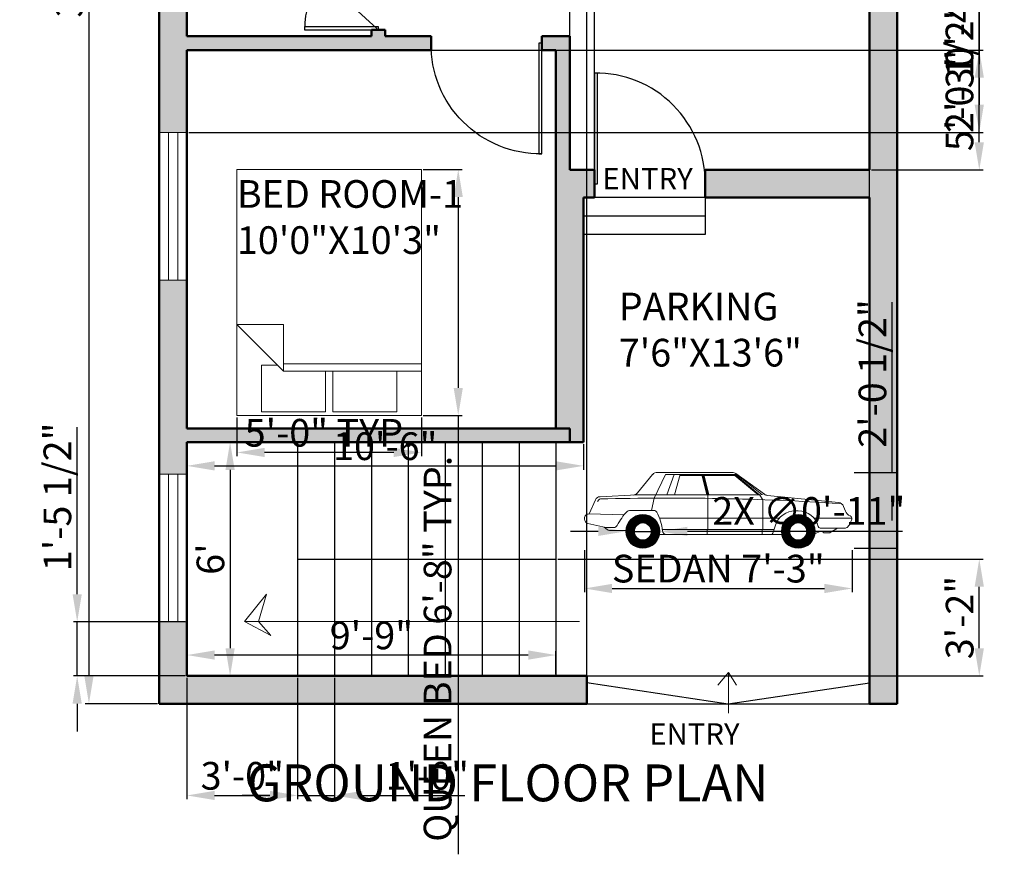
# Model space of a CAD drawing. Units: inches. Extents: x 66818 to 67138, y 29633 to 30215.
# Tile 1 of 2: x 66818 to 67138, y 29633 to 29904. Entities that reach past the tile are written whole.
import ezdxf

# ---------------------------------------------------------------- set-up
doc = ezdxf.new("R2010")
doc.units = ezdxf.units.IN
for name, color, linetype, lineweight in [('A-ANNO-DIMS', 2, 'Continuous', 18), ('A-ANNO-SYMB', 7, 'Continuous', 18), ('A-ANNO-TEXT', 7, 'Continuous', 25), ('A-AREA-IDEN', 7, 'Continuous', 25), ('A-DOOR', 3, 'Continuous', 25), ('A-FLOR-STRS', 7, 'Continuous', 25), ('A-FURN', 8, 'Continuous', 18), ('A-GLAZ', 4, 'Continuous', 18), ('A-SITE-PARK', 9, 'Continuous', 13), ('A-WALL', 7, 'Continuous', 50)]:
    doc.layers.add(name, color=color, linetype=linetype, lineweight=lineweight)
doc.layers.add('A-WALL-PATT', color=251, linetype='Continuous', lineweight=13, true_color=0x636466)
doc.styles.get("Standard").update_dxf_attribs({"font": 'arial.ttf'})
doc.dimstyles.new('ISO-25', dxfattribs={"dimtxt": 9, "dimasz": 9, "dimexe": 1.25, "dimexo": 0.625, "dimtad": 1, "dimdec": 1, "dimrnd": 9, "dimlunit": 3, "dimtxsty": 'Standard', "dimcen": 2.5, "dimadec": 0, "dimazin": 0, "dimtfac": 1, "dimtdec": 1, "dimtmove": 0, "dimatfit": 3, "dimfxl": 1, "dimarcsym": 0})

# ---------------------------------------------------------------- blocks, each defined once
blk = doc.blocks.new('*D1')
at = {"layer": 'A-ANNO-DIMS', "color": 0, "lineweight": -2, "transparency": 16777216}
for p, q in [((66872.23, 29766.29), (66872.23, 29757.97)), ((67001.23, 29766.29), (67001.23, 29757.97)), ((66881.23, 29759.22), (66992.23, 29759.22))]:
    blk.add_line(p, q, dxfattribs=at)
at = {"layer": 'A-ANNO-DIMS', "color": 0, "transparency": 16777216}
for points in [[(66881.23, 29760.72), (66881.23, 29757.72), (66872.23, 29759.22)], [(66992.23, 29760.72), (66992.23, 29757.72), (67001.23, 29759.22)]]:
    blk.add_solid(points, dxfattribs=at)
at = {"layer": 'Defpoints', "color": 0, "transparency": 16777216}
for p in [(66872.23, 29766.91), (67001.23, 29766.91), (67001.23, 29759.22)]:
    blk.add_point(p, dxfattribs=at)
at = {"layer": 'A-ANNO-DIMS', "color": 0, "transparency": 16777216, "insert": (66936.73, 29764.44), "char_height": 9, "attachment_point": 5}
blk.add_mtext('10\'-6"', dxfattribs=at)
blk = doc.blocks.new('*D2')
at = {"layer": 'A-ANNO-DIMS', "color": 0, "lineweight": -2, "transparency": 16777216}
for p, q in [((66872.85, 29766.91), (66887.51, 29766.91)), ((66886.26, 29757.91), (66886.26, 29699.91)), ((66872.85, 29690.91), (66887.51, 29690.91))]:
    blk.add_line(p, q, dxfattribs=at)
at = {"layer": 'A-ANNO-DIMS', "color": 0, "transparency": 16777216}
for points in [[(66884.76, 29757.91), (66887.76, 29757.91), (66886.26, 29766.91)], [(66884.76, 29699.91), (66887.76, 29699.91), (66886.26, 29690.91)]]:
    blk.add_solid(points, dxfattribs=at)
at = {"layer": 'Defpoints', "color": 0, "transparency": 16777216}
for p in [(66872.23, 29766.91), (66872.23, 29690.91), (66886.26, 29690.91)]:
    blk.add_point(p, dxfattribs=at)
at = {"layer": 'A-ANNO-DIMS', "color": 0, "transparency": 16777216, "insert": (66881.04, 29728.91), "char_height": 9, "attachment_point": 5, "rotation": 90}
blk.add_mtext("6'", dxfattribs=at)
blk = doc.blocks.new('*D3')
at = {"layer": 'A-ANNO-DIMS', "color": 0, "lineweight": -2, "transparency": 16777216}
for p, q in [((66872.23, 29691.54), (66872.23, 29698.96)), ((66983.23, 29697.71), (66881.23, 29697.71)), ((66992.23, 29691.54), (66992.23, 29698.96))]:
    blk.add_line(p, q, dxfattribs=at)
at = {"layer": 'A-ANNO-DIMS', "color": 0, "transparency": 16777216}
for points in [[(66881.23, 29699.21), (66881.23, 29696.21), (66872.23, 29697.71)], [(66983.23, 29699.21), (66983.23, 29696.21), (66992.23, 29697.71)]]:
    blk.add_solid(points, dxfattribs=at)
at = {"layer": 'Defpoints', "color": 0, "transparency": 16777216}
for p in [(66872.23, 29697.71), (66872.23, 29690.91), (66992.23, 29690.91)]:
    blk.add_point(p, dxfattribs=at)
at = {"layer": 'A-ANNO-DIMS', "color": 0, "transparency": 16777216, "insert": (66932.23, 29702.93), "char_height": 9, "attachment_point": 5}
blk.add_mtext('9\'-9"', dxfattribs=at)
blk = doc.blocks.new('Bed - Queen')
for p, q in [((0, -80.00003), (0, 0)), ((0, 0), (59.99999, 0)), ((59.99999, 0), (59.99999, -80.00003)), ((7.99999, -1.2), (28.79998, -1.2)), ((7.99999, -14.4), (7.99999, -1.2)), ((28.79998, -1.2), (28.79998, -14.4)), ((31.19999, -1.2), (51.99999, -1.2)), ((31.19999, -14.4), (31.19999, -1.2)), ((51.99999, -1.2), (51.99999, -16.4)), ((0, -14.4), (44.8, -14.4)), ((59.99999, -29.6), (44.8, -14.4)), ((44.8, -14.4), (44.8, -29.6)), ((44.8, -16.8), (0, -16.8)), ((51.99999, -16.4), (46.79936, -16.4)), ((44.8, -29.6), (59.99999, -29.6)), ((59.99999, -80.00003), (0, -80.00003))]:
    blk.add_line(p, q)
blk = doc.blocks.new('Car - sedan  side')
for p, q in [((-139.53, 35.99), (-129.64, 47.91)), ((-128.57, 32.64), (-121.22, 48.02)), ((-77.81, 49.34), (-126.58, 49.34)), ((-74.7, 48.02), (-121.22, 48.02)), ((-120.32, 34.67), (-115.67, 48.02)), ((-115.4, 34.67), (-111.74, 48.02)), ((-97.55, 47.3), (-111.94, 47.3)), ((-94.41, 34.67), (-97.73, 48.02)), ((-93.72, 34.67), (-97.04, 48.02)), ((-93.03, 34.67), (-96.34, 48.02)), ((-76.26, 47.3), (-96.16, 47.3)), ((-61.08, 34.66), (-76.26, 47.3)), ((-60.02, 34.65), (-76.07, 48.02)), ((-56.87, 35.13), (-75.48, 48.59)), ((-58.54, 34.93), (-74.99, 48.02)), ((-140.23, 34.67), (-163.88, 33.56)), ((-62.28, 34.67), (-140.23, 34.67)), ((-130.39, 24.63), (-128.57, 32.64)), ((-93.72, 19.62), (-93.72, 34.67)), ((-62.28, 34.67), (-60.02, 34.65)), ((-60.02, 34.65), (-58.54, 34.93)), ((-57.97, 31.61), (-60.02, 34.65)), ((-57.21, 35.38), (-58.54, 34.93)), ((-54.93, 34.4), (-8.75, 29.8)), ((-170.93, 22.32), (-166.81, 31.56)), ((-164.57, 31.6), (-165.48, 30.35)), ((-57.97, 19.62), (-57.97, 31.61)), ((-4.21, 24.18), (-5.42, 27.27)), ((-174, 19.51), (-174, 18.91)), ((-148.26, 21.7), (-171.11, 22.33)), ((-128.78, 24.63), (-144.79, 24.63)), ((-47.2, 19.62), (-125.23, 19.62)), ((-93.72, 12.14), (-93.72, 19.62)), ((-57.97, 12.14), (-57.97, 19.62)), ((-36.97, 24.38), (-34.94, 24.38)), ((0, 19.62), (-24.7, 19.62)), ((-160.12, 13.48), (-171.81, 16.16)), ((-159.22, 12.14), (-161.08, 13.7)), ((-155.01, 13.48), (-160.12, 13.48)), ((-51.4, 9.89), (-49.69, 15.14)), ((-4.23, 13.19), (-20.72, 13.19)), ((-9.5, 13.19), (-14.1, 10.2)), ((-3.22, 13.59), (-1.77, 14.97)), ((-147.03, 11.6), (-157.73, 11.6)), ((-120.62, 9.03), (-125.23, 9.03)), ((-50.67, 12.14), (-123.32, 12.14)), ((-45.76, 9.03), (-120.62, 9.03)), ((-94.21, 9.03), (-94.21, 12.14)), ((-58.39, 9.03), (-58.39, 12.14)), ((-20.36, 11.06), (-24.06, 9.44)), ((-18.83, 10.42), (-19.11, 10.76)), ((-14.68, 10.03), (-18.01, 10.03))]:
    blk.add_line(p, q)
at = {"const_width": 5.49}
for points in [[(-127.8, 11, -1), (-144.3, 11, -1)], [(-26.69, 11, -1), (-43.19, 11, -1)]]:
    blk.add_lwpolyline(points, format="xyb", close=True, dxfattribs=at)
for centre, radius in [((-136.05, 11), 11), ((-34.94, 11), 11), ((-136.05, 11), 5.51), ((-34.94, 11), 5.51)]:
    blk.add_circle(centre, radius)
for centre, radius, start, end in [((-126.58, 45.38), 3.97, 90, 140.30288), ((-77.81, 45.38), 3.97, 54.13504, 90), ((-163.72, 30.18), 3.38, 92.68266, 155.97362), ((-163.62, 30.91), 1.17, 91.49105, 143.95527), ((-118.51, -1702.12), 1734.79, 86.34698, 91.49105), ((-142.58, 38.53), 3.97, 272.68265, 320.30288), ((-54.54, 38.35), 3.97, 234.13503, 264.31231), ((-9.15, 25.82), 4, 21.31069, 84.3123), ((-171.18, 19.51), 2.82, 88.41927, 180), ((-118.09, -2.78), 38.85, 136.3964, 152.90974), ((-144.79, 22.64), 1.98, 90, 136.3964), ((-128.78, 22.64), 1.98, 28.1371, 90), ((-157.14, 7.48), 34.14, 6.51354, 28.1371), ((-36.97, 11), 13.38, 90, 161.97316), ((-34.94, 11), 13.38, 13.58642, 90), ((0.9, 26.18), 5.49, 201.3107, 247.70484), ((-1.92, 19.3), 1.94, 325.37436, 67.70485), ((-171.18, 18.91), 2.82, 180, 257.09053), ((-155.01, 16.1), 2.62, 270, 332.90974), ((-20.72, 14.43), 1.24, 193.58641, 270), ((-4.23, 14.65), 1.46, 270, 313.71735), ((-3.82, 17.12), 2.96, 313.71735, 352.38387), ((2.46, 16.28), 3.37, 145.37437, 172.38386), ((-157.73, 13.93), 2.32, 230.12913, 270), ((-120.62, 11.65), 2.62, 186.51353, 270), ((-52.58, 10.27), 1.24, 270, 341.97316), ((-19.93, 10.09), 1.06, 39.30103, 113.71592), ((-18.01, 11.09), 1.06, 219.30104, 270), ((-14.68, 11.09), 1.06, 270, 303.04697)]:
    blk.add_arc(centre, radius, start, end)
blk = doc.blocks.new('*D10')
at = {"layer": 'A-ANNO-DIMS', "color": 0, "lineweight": -2, "transparency": 16777216}
for p, q in [((66862.6, 30161.91), (66839.1, 30161.91)), ((66840.35, 30152.91), (66840.35, 29690.91)), ((66862.6, 29681.91), (66839.1, 29681.91))]:
    blk.add_line(p, q, dxfattribs=at)
at = {"layer": 'A-ANNO-DIMS', "color": 0, "transparency": 16777216}
for points in [[(66838.85, 30152.91), (66841.85, 30152.91), (66840.35, 30161.91)], [(66838.85, 29690.91), (66841.85, 29690.91), (66840.35, 29681.91)]]:
    blk.add_solid(points, dxfattribs=at)
at = {"layer": 'Defpoints', "color": 0, "transparency": 16777216}
for p in [(66863.23, 30161.91), (66840.35, 29681.91), (66863.23, 29681.91)]:
    blk.add_point(p, dxfattribs=at)
at = {"layer": 'A-ANNO-DIMS', "color": 0, "transparency": 16777216, "insert": (66835.13, 29921.91), "char_height": 9, "attachment_point": 5, "rotation": 90}
blk.add_mtext('39\'-9"', dxfattribs=at)
blk = doc.blocks.new('WIN-48IN')
for p, q in [((9, 48), (0, 48)), ((3, 48), (3, 0)), ((6, 48), (6, 0)), ((9, 0), (0, 0))]:
    blk.add_line(p, q)
blk = doc.blocks.new('DOOR-SWING-36IN')
for p, q in [((35, 0), (35, 36)), ((35, 36), (36, 36)), ((36, 36), (36, 2.25)), ((36, 0), (35, 0))]:
    blk.add_line(p, q)
blk.add_arc((35.5, 0.5), 35.5, 89.1931, 180.8069)
blk = doc.blocks.new('*D15')
at = {"layer": 'A-ANNO-DIMS', "color": 0, "lineweight": -2, "transparency": 16777216}
for p, q in [((66949.09, 29855.58), (66961.72, 29855.58)), ((66960.47, 29846.58), (66960.47, 29784.58)), ((66949.09, 29775.58), (66961.72, 29775.58)), ((66960.47, 29775.58), (66960.47, 29632.94))]:
    blk.add_line(p, q, dxfattribs=at)
at = {"layer": 'A-ANNO-DIMS', "color": 0, "transparency": 16777216}
for points in [[(66958.97, 29846.58), (66961.97, 29846.58), (66960.47, 29855.58)], [(66958.97, 29784.58), (66961.97, 29784.58), (66960.47, 29775.58)]]:
    blk.add_solid(points, dxfattribs=at)
at = {"layer": 'Defpoints', "color": 0, "transparency": 16777216}
for p in [(66948.47, 29855.58), (66948.47, 29775.58), (66960.47, 29775.58)]:
    blk.add_point(p, dxfattribs=at)
at = {"layer": 'A-ANNO-DIMS', "color": 0, "transparency": 16777216, "insert": (66954.91, 29699.76), "char_height": 9, "attachment_point": 5, "rotation": 90}
blk.add_mtext('QUEEN BED 6\'-8" TYP.', dxfattribs=at)
blk = doc.blocks.new('*D16')
at = {"layer": 'A-ANNO-DIMS', "color": 0, "lineweight": -2, "transparency": 16777216}
for p, q in [((66888.47, 29774.96), (66888.47, 29762.33)), ((66948.47, 29774.96), (66948.47, 29762.33)), ((66939.47, 29763.58), (66897.47, 29763.58))]:
    blk.add_line(p, q, dxfattribs=at)
at = {"layer": 'A-ANNO-DIMS', "color": 0, "transparency": 16777216}
for points in [[(66897.47, 29765.08), (66897.47, 29762.08), (66888.47, 29763.58)], [(66939.47, 29765.08), (66939.47, 29762.08), (66948.47, 29763.58)]]:
    blk.add_solid(points, dxfattribs=at)
at = {"layer": 'Defpoints', "color": 0, "transparency": 16777216}
for p in [(66888.47, 29775.58), (66948.47, 29775.58), (66888.47, 29763.58)]:
    blk.add_point(p, dxfattribs=at)
at = {"layer": 'A-ANNO-DIMS', "color": 0, "transparency": 16777216, "insert": (66918.47, 29768.8), "char_height": 9, "attachment_point": 5}
blk.add_mtext('5\'-0" TYP.', dxfattribs=at)
blk = doc.blocks.new('*D25')
at = {"layer": 'A-ANNO-DIMS', "color": 0, "lineweight": -2, "transparency": 16777216}
for p, q in [((67001.52, 29731.79), (67001.52, 29718.11)), ((67088.57, 29731.79), (67088.57, 29718.11)), ((67010.52, 29719.36), (67079.57, 29719.36))]:
    blk.add_line(p, q, dxfattribs=at)
at = {"layer": 'A-ANNO-DIMS', "color": 0, "transparency": 16777216}
for points in [[(67010.52, 29720.86), (67010.52, 29717.86), (67001.52, 29719.36)], [(67079.57, 29720.86), (67079.57, 29717.86), (67088.57, 29719.36)]]:
    blk.add_solid(points, dxfattribs=at)
at = {"layer": 'Defpoints', "color": 0, "transparency": 16777216}
for p in [(67001.52, 29732.42), (67088.57, 29732.42), (67088.57, 29719.36)]:
    blk.add_point(p, dxfattribs=at)
at = {"layer": 'A-ANNO-DIMS', "color": 0, "transparency": 16777216, "insert": (67045.04, 29724.64), "char_height": 9, "attachment_point": 5}
blk.add_mtext('SEDAN 7\'-3"', dxfattribs=at)
blk = doc.blocks.new('*D26')
at = {"layer": 'A-ANNO-DIMS', "color": 0, "lineweight": -2, "transparency": 16777216}
for p, q in [((67101.63, 29757.09), (67101.63, 29812.39)), ((67089.2, 29757.09), (67102.88, 29757.09)), ((67101.63, 29741.42), (67101.63, 29748.09)), ((67089.2, 29732.42), (67102.88, 29732.42))]:
    blk.add_line(p, q, dxfattribs=at)
at = {"layer": 'A-ANNO-DIMS', "color": 0, "transparency": 16777216}
for points in [[(67100.13, 29748.09), (67103.13, 29748.09), (67101.63, 29757.09)], [(67100.13, 29741.42), (67103.13, 29741.42), (67101.63, 29732.42)]]:
    blk.add_solid(points, dxfattribs=at)
at = {"layer": 'Defpoints', "color": 0, "transparency": 16777216}
for p in [(67088.57, 29757.09), (67101.63, 29757.09), (67088.57, 29732.42)]:
    blk.add_point(p, dxfattribs=at)
at = {"layer": 'A-ANNO-DIMS', "color": 0, "transparency": 16777216, "insert": (67096.35, 29789.24), "char_height": 9, "attachment_point": 5, "rotation": 90}
blk.add_mtext('2\'-0 1/2"', dxfattribs=at)
blk = doc.blocks.new('*D29')
at = {"layer": 'A-ANNO-DIMS', "color": 0, "lineweight": -2, "transparency": 16777216}
for p, q in [((67129.93, 29967.41), (67129.93, 29976.41)), ((66932.85, 29958.41), (67131.18, 29958.41)), ((67129.93, 29958.41), (67129.93, 29953.91)), ((66932.85, 29953.91), (67131.18, 29953.91)), ((67129.93, 29944.91), (67129.93, 29889.77))]:
    blk.add_line(p, q, dxfattribs=at)
at = {"layer": 'A-ANNO-DIMS', "color": 0, "transparency": 16777216}
for points in [[(67128.43, 29967.41), (67131.43, 29967.41), (67129.93, 29958.41)], [(67128.43, 29944.91), (67131.43, 29944.91), (67129.93, 29953.91)]]:
    blk.add_solid(points, dxfattribs=at)
at = {"layer": 'Defpoints', "color": 0, "transparency": 16777216}
for p in [(66932.23, 29958.41), (66932.23, 29953.91), (67129.93, 29953.91)]:
    blk.add_point(p, dxfattribs=at)
at = {"layer": 'A-ANNO-DIMS', "color": 0, "transparency": 16777216, "insert": (67124.65, 29912.84), "char_height": 9, "attachment_point": 5, "rotation": 90}
blk.add_mtext('0\'-4 1/2"', dxfattribs=at)
blk = doc.blocks.new('*D32')
at = {"layer": 'A-ANNO-DIMS', "color": 0, "lineweight": -2, "transparency": 16777216}
for p, q in [((67094.85, 29915.99), (67131.18, 29915.99)), ((67129.93, 29864.41), (67129.93, 29906.99)), ((67094.85, 29855.41), (67131.18, 29855.41))]:
    blk.add_line(p, q, dxfattribs=at)
at = {"layer": 'A-ANNO-DIMS', "color": 0, "transparency": 16777216}
for points in [[(67128.43, 29906.99), (67131.43, 29906.99), (67129.93, 29915.99)], [(67128.43, 29864.41), (67131.43, 29864.41), (67129.93, 29855.41)]]:
    blk.add_solid(points, dxfattribs=at)
at = {"layer": 'Defpoints', "color": 0, "transparency": 16777216}
for p in [(67094.23, 29915.99), (67129.93, 29915.99), (67094.23, 29855.41)]:
    blk.add_point(p, dxfattribs=at)
at = {"layer": 'A-ANNO-DIMS', "color": 0, "transparency": 16777216, "insert": (67124.65, 29885.7), "char_height": 9, "attachment_point": 5, "rotation": 90}
blk.add_mtext('5\'-0 1/2"', dxfattribs=at)
blk = doc.blocks.new('*D35')
at = {"layer": 'A-ANNO-DIMS', "color": 0, "lineweight": -2, "transparency": 16777216}
for p, q in [((66872.85, 29894.41), (67131.18, 29894.41)), ((67129.93, 29885.41), (67129.93, 29876.61)), ((66872.85, 29867.61), (67131.18, 29867.61))]:
    blk.add_line(p, q, dxfattribs=at)
at = {"layer": 'A-ANNO-DIMS', "color": 0, "transparency": 16777216}
for points in [[(67128.43, 29885.41), (67131.43, 29885.41), (67129.93, 29894.41)], [(67128.43, 29876.61), (67131.43, 29876.61), (67129.93, 29867.61)]]:
    blk.add_solid(points, dxfattribs=at)
at = {"layer": 'Defpoints', "color": 0, "transparency": 16777216}
for p in [(66872.23, 29894.41), (66872.23, 29867.61), (67129.93, 29867.61)]:
    blk.add_point(p, dxfattribs=at)
at = {"layer": 'A-ANNO-DIMS', "color": 0, "transparency": 16777216, "insert": (67124.71, 29881.01), "char_height": 9, "attachment_point": 5, "rotation": 90}
blk.add_mtext('2\'-3"', dxfattribs=at)
blk = doc.blocks.new('*D36')
at = {"layer": 'A-ANNO-DIMS', "color": 0, "lineweight": -2, "transparency": 16777216}
for p, q in [((66836.53, 29717.49), (66836.53, 29771.78)), ((66871.6, 29708.49), (66835.28, 29708.49)), ((66836.53, 29690.91), (66836.53, 29708.49)), ((66871.6, 29690.91), (66835.28, 29690.91)), ((66836.53, 29681.91), (66836.53, 29672.91))]:
    blk.add_line(p, q, dxfattribs=at)
at = {"layer": 'A-ANNO-DIMS', "color": 0, "transparency": 16777216}
for points in [[(66835.03, 29717.49), (66838.03, 29717.49), (66836.53, 29708.49)], [(66835.03, 29681.91), (66838.03, 29681.91), (66836.53, 29690.91)]]:
    blk.add_solid(points, dxfattribs=at)
at = {"layer": 'Defpoints', "color": 0, "transparency": 16777216}
for p in [(66836.53, 29708.49), (66872.23, 29708.49), (66872.23, 29690.91)]:
    blk.add_point(p, dxfattribs=at)
at = {"layer": 'A-ANNO-DIMS', "color": 0, "transparency": 16777216, "insert": (66831.25, 29749.14), "char_height": 9, "attachment_point": 5, "rotation": 90}
blk.add_mtext('1\'-5 1/2"', dxfattribs=at)
blk = doc.blocks.new('*D37')
at = {"layer": 'A-ANNO-DIMS', "color": 0, "lineweight": -2, "transparency": 16777216}
for p, q in [((66872.23, 29690.29), (66872.23, 29650.82)), ((66908.23, 29690.29), (66908.23, 29650.82)), ((66881.23, 29652.07), (66899.23, 29652.07))]:
    blk.add_line(p, q, dxfattribs=at)
at = {"layer": 'A-ANNO-DIMS', "color": 0, "transparency": 16777216}
for points in [[(66881.23, 29653.57), (66881.23, 29650.57), (66872.23, 29652.07)], [(66899.23, 29653.57), (66899.23, 29650.57), (66908.23, 29652.07)]]:
    blk.add_solid(points, dxfattribs=at)
at = {"layer": 'Defpoints', "color": 0, "transparency": 16777216}
for p in [(66872.23, 29690.91), (66908.23, 29690.91), (66908.23, 29652.07)]:
    blk.add_point(p, dxfattribs=at)
at = {"layer": 'A-ANNO-DIMS', "color": 0, "transparency": 16777216, "insert": (66890.23, 29657.29), "char_height": 9, "attachment_point": 5}
blk.add_mtext('3\'-0"', dxfattribs=at)
blk = doc.blocks.new('*D38')
at = {"layer": 'A-ANNO-DIMS', "color": 0, "lineweight": -2, "transparency": 16777216}
for p, q in [((66908.23, 29690.29), (66908.23, 29650.82)), ((66920.23, 29690.29), (66920.23, 29650.82)), ((66899.23, 29652.07), (66890.23, 29652.07)), ((66908.23, 29652.07), (66920.23, 29652.07)), ((66929.23, 29652.07), (66962.56, 29652.07))]:
    blk.add_line(p, q, dxfattribs=at)
at = {"layer": 'A-ANNO-DIMS', "color": 0, "transparency": 16777216}
for points in [[(66899.23, 29653.57), (66899.23, 29650.57), (66908.23, 29652.07)], [(66929.23, 29653.57), (66929.23, 29650.57), (66920.23, 29652.07)]]:
    blk.add_solid(points, dxfattribs=at)
at = {"layer": 'Defpoints', "color": 0, "transparency": 16777216}
for p in [(66908.23, 29690.91), (66920.23, 29690.91), (66920.23, 29652.07)]:
    blk.add_point(p, dxfattribs=at)
at = {"layer": 'A-ANNO-DIMS', "color": 0, "transparency": 16777216, "insert": (66950.39, 29657.29), "char_height": 9, "attachment_point": 5}
blk.add_mtext('1\'-0"', dxfattribs=at)
blk = doc.blocks.new('*D39')
at = {"layer": 'A-ANNO-DIMS', "color": 0, "lineweight": -2, "transparency": 16777216}
for p, q in [((66992.85, 29728.91), (67131.18, 29728.91)), ((67129.93, 29699.91), (67129.93, 29719.91)), ((66992.85, 29690.91), (67131.18, 29690.91))]:
    blk.add_line(p, q, dxfattribs=at)
at = {"layer": 'A-ANNO-DIMS', "color": 0, "transparency": 16777216}
for points in [[(67128.43, 29719.91), (67131.43, 29719.91), (67129.93, 29728.91)], [(67128.43, 29699.91), (67131.43, 29699.91), (67129.93, 29690.91)]]:
    blk.add_solid(points, dxfattribs=at)
at = {"layer": 'Defpoints', "color": 0, "transparency": 16777216}
for p in [(66992.23, 29728.91), (67129.93, 29728.91), (66992.23, 29690.91)]:
    blk.add_point(p, dxfattribs=at)
at = {"layer": 'A-ANNO-DIMS', "color": 0, "transparency": 16777216, "insert": (67124.71, 29709.91), "char_height": 9, "attachment_point": 5, "rotation": 90}
blk.add_mtext('3\'-2"', dxfattribs=at)
blk = doc.blocks.new('*D43')
at = {"layer": 'A-ANNO-DIMS', "color": 0, "lineweight": -2, "transparency": 16777216}
for p, q in [((67002.34, 29682.54), (67002.34, 30189.86)), ((67094.23, 29682.54), (67094.23, 30189.86)), ((67011.34, 30188.61), (67085.23, 30188.61))]:
    blk.add_line(p, q, dxfattribs=at)
at = {"layer": 'A-ANNO-DIMS', "color": 0, "transparency": 16777216}
for points in [[(67011.34, 30190.11), (67011.34, 30187.11), (67002.34, 30188.61)], [(67085.23, 30190.11), (67085.23, 30187.11), (67094.23, 30188.61)]]:
    blk.add_solid(points, dxfattribs=at)
at = {"layer": 'Defpoints', "color": 0, "transparency": 16777216}
for p in [(67094.23, 30188.61), (67002.34, 29681.91), (67094.23, 29681.91)]:
    blk.add_point(p, dxfattribs=at)
at = {"layer": 'A-ANNO-DIMS', "color": 0, "transparency": 16777216, "insert": (67048.28, 30193.83), "char_height": 9, "attachment_point": 5}
blk.add_mtext('7\'-8"', dxfattribs=at)
blk = doc.blocks.new('*D44')
at = {"layer": 'A-ANNO-DIMS', "color": 0, "lineweight": -2, "transparency": 16777216}
for p, q in [((66996.73, 29856.04), (66996.73, 30189.86)), ((67004.76, 29856.04), (67004.76, 30189.86)), ((66987.73, 30188.61), (66978.73, 30188.61)), ((66996.73, 30188.61), (67004.76, 30188.61)), ((67013.76, 30188.61), (67047.94, 30188.61))]:
    blk.add_line(p, q, dxfattribs=at)
at = {"layer": 'A-ANNO-DIMS', "color": 0, "transparency": 16777216}
for points in [[(66987.73, 30190.11), (66987.73, 30187.11), (66996.73, 30188.61)], [(67013.76, 30190.11), (67013.76, 30187.11), (67004.76, 30188.61)]]:
    blk.add_solid(points, dxfattribs=at)
at = {"layer": 'Defpoints', "color": 0, "transparency": 16777216}
for p in [(67004.76, 30188.61), (66996.73, 29855.41), (67004.76, 29855.41)]:
    blk.add_point(p, dxfattribs=at)
at = {"layer": 'A-ANNO-DIMS', "color": 0, "transparency": 16777216, "insert": (67035.35, 30193.83), "char_height": 9, "attachment_point": 5}
blk.add_mtext('0\'-8"', dxfattribs=at)
blk = doc.blocks.new('*D46')
at = {"layer": 'A-ANNO-DIMS', "color": 0, "lineweight": -2, "transparency": 16777216}
for p, q in [((66843.04, 29983.89), (66909.91, 29923.29)), ((66934.04, 29901.42), (66916.58, 29917.25))]:
    blk.add_line(p, q, dxfattribs=at)
at = {"layer": 'A-ANNO-DIMS', "color": 0, "transparency": 16777216}
blk.add_solid([(66910.92, 29924.4), (66908.9, 29922.18), (66916.58, 29917.25)], dxfattribs=at)
at = {"layer": 'Defpoints', "color": 0, "transparency": 16777216}
for p in [(66916.58, 29917.25), (66934.04, 29901.42)]:
    blk.add_point(p, dxfattribs=at)
at = {"layer": 'A-ANNO-DIMS', "color": 0, "transparency": 16777216, "insert": (66876.69, 29960.52), "char_height": 9, "attachment_point": 5, "rotation": 317.8154}
blk.add_mtext('2X R1\'-11 1/2"', dxfattribs=at)
blk = doc.blocks.new('*D47')
at = {"layer": 'A-ANNO-DIMS', "color": 0, "lineweight": -2, "transparency": 16777216}
for p, q in [((67005.99, 29737.92), (66996.99, 29737.92)), ((67014.99, 29737.92), (67025.99, 29737.92)), ((67104.96, 29737.92), (67034.99, 29737.92))]:
    blk.add_line(p, q, dxfattribs=at)
at = {"layer": 'A-ANNO-DIMS', "color": 0, "transparency": 16777216}
for points in [[(67005.99, 29739.42), (67005.99, 29736.42), (67014.99, 29737.92)], [(67034.99, 29739.42), (67034.99, 29736.42), (67025.99, 29737.92)]]:
    blk.add_solid(points, dxfattribs=at)
at = {"layer": 'Defpoints', "color": 0, "transparency": 16777216}
for p in [(67014.99, 29737.92), (67025.99, 29737.92)]:
    blk.add_point(p, dxfattribs=at)
at = {"layer": 'A-ANNO-DIMS', "color": 0, "transparency": 16777216, "insert": (67074.48, 29743.39), "char_height": 9, "attachment_point": 5, "rotation": 0.003}
blk.add_mtext('2X ∅0\'-11"', dxfattribs=at)

msp = doc.modelspace()

# ---------------------------------------------------------------- hatches: boundary and pattern name
at = {"layer": 'A-WALL-PATT'}
h = msp.add_hatch(color=256, dxfattribs=at)
h.dxf.hatch_style = 1
h.paths.add_polyline_path([(66872.23, 30152.91), (66992.23, 30152.91), (66992.23, 30022.91), (66990.58, 30022.91), (66990.58, 30018.41), (66998.73, 30018.41), (66998.73, 30022.91), (66996.73, 30022.91), (66996.73, 30152.91), (67094.23, 30152.91), (67094.23, 30111.23), (67103.23, 30111.23), (67103.23, 30161.91), (66863.23, 30161.91), (66863.23, 30117.42), (66872.23, 30117.42)])
h.paths.add_polyline_path([(66872.23, 30069.42), (66863.23, 30069.42), (66863.23, 29990.63), (66872.23, 29990.63), (66872.23, 30018.41), (66877.23, 30018.41), (66877.23, 30022.91), (66872.23, 30022.91)])
h.paths.add_polyline_path([(66954.58, 30020.66, -0.007042), (66954.58, 30021.66), (66954.58, 30022.91), (66901.23, 30022.91), (66901.23, 30020.66, -0.010637), (66901.23, 30019.66), (66901.23, 30018.41), (66932.23, 30018.41), (66932.23, 29958.41), (66872.23, 29958.41), (66872.23, 29966.63), (66863.23, 29966.63), (66863.23, 29867.61), (66872.23, 29867.61), (66872.23, 29894.41), (66951.63, 29894.41), (66951.63, 29895.66, -0.007042), (66951.63, 29896.66), (66951.63, 29898.91), (66936.73, 29898.91), (66936.73, 29900.92), (66932.23, 29900.92), (66932.23, 29898.91), (66872.23, 29898.91), (66872.23, 29953.91), (66932.23, 29953.91), (66932.23, 29924.92), (66936.73, 29924.92), (66936.73, 30018.41), (66954.58, 30018.41)])
h.paths.add_polyline_path([(67103.23, 30063.23), (67094.23, 30063.23), (67094.23, 30022.91), (67034.78, 30022.91, -0.031636), (67034.73, 30018.41), (67094.23, 30018.41), (67094.23, 29963.99), (67103.23, 29963.99)])
h.paths.add_polyline_path([(67103.23, 29915.99), (67094.23, 29915.99), (67094.23, 29855.41), (67040.76, 29855.41), (67040.76, 29851.91, -0.007042), (67040.76, 29850.91), (67040.76, 29846.41), (67094.23, 29846.41), (67094.23, 29690.91), (67094.23, 29681.91), (67103.23, 29681.91)])
h.paths.add_polyline_path([(67001.23, 29846.41), (67004.76, 29846.41), (67004.76, 29855.41), (66996.73, 29855.41), (66996.73, 29898.91), (66987.63, 29898.91), (66987.63, 29894.41), (66992.23, 29894.41), (66992.23, 29771.41), (66996.73, 29771.41), (66996.73, 29766.91), (67001.23, 29766.91), (67001.23, 29771.41)])
h.paths.add_polyline_path([(66872.23, 29819.61), (66863.23, 29819.61), (66863.23, 29756.49), (66872.23, 29756.49), (66872.23, 29766.91), (66996.73, 29766.91), (66996.73, 29771.41), (66872.23, 29771.41)])
h.paths.add_polyline_path([(67002.34, 29690.91), (66872.23, 29690.91), (66872.23, 29708.49), (66863.23, 29708.49), (66863.23, 29681.91), (67002.34, 29681.91)])
h.paths.add_polyline_path([(66918.07, 29755.08), (66954.6, 29755.08), (66954.6, 29773.63), (66918.07, 29773.63)], flags=9)

# ---------------------------------------------------------------- linework, layer by layer
at = {"layer": 'A-ANNO-SYMB'}
for p, q in [((66890.91, 29708.65), (66898.14, 29717.48)), ((66898.14, 29717.48), (66895.46, 29708.65)), ((66999.86, 29708.65), (66890.91, 29708.65)), ((66899.48, 29704.11), (66890.91, 29708.65)), ((66895.46, 29708.65), (66899.48, 29704.11)), ((67048.37, 29692.09), (67044.88, 29687.91)), ((67048.37, 29678.77), (67048.37, 29692.09)), ((67048.37, 29692.09), (67051.01, 29687.91))]:
    msp.add_line(p, q, dxfattribs=at)
at = {"layer": 'A-DOOR'}
for p, q in [((66934.48, 29901.92), (66910.48, 29901.92)), ((66910.48, 29901.92), (66910.48, 29900.92)), ((66934.48, 29900.92), (66934.48, 29901.92)), ((66910.48, 29900.92), (66932.23, 29900.92)), ((67005.76, 29886.91), (67004.76, 29886.91)), ((67004.76, 29886.91), (67004.76, 29855.41)), ((67005.76, 29850.91), (67005.76, 29886.91)), ((67004.76, 29850.91), (67005.76, 29850.91)), ((67002.34, 29688.82), (67048.28, 29681.91)), ((67048.28, 29681.91), (67094.23, 29688.68)), ((67002.34, 29681.91), (67094.23, 29681.91))]:
    msp.add_line(p, q, dxfattribs=at)
for centre, radius, start, end in [((66934.04, 29901.42), 23.57, 94.4156, 181.2155), ((67005.26, 29851.41), 35.5, 359.1931, 90.8069)]:
    msp.add_arc(centre, radius, start, end, dxfattribs=at)
at = {"layer": 'A-FLOR-STRS'}
for p, q in [((67040.76, 29846.41), (67001.23, 29846.41)), ((67040.76, 29846.41), (67040.76, 29834.41)), ((67040.76, 29840.41), (67001.23, 29840.41)), ((67040.76, 29834.41), (67001.23, 29834.41)), ((66908.23, 29766.91), (66908.23, 29690.91)), ((66920.23, 29766.91), (66920.23, 29690.91)), ((66932.23, 29766.91), (66932.23, 29690.91)), ((66944.23, 29766.91), (66944.23, 29690.91)), ((66956.23, 29766.91), (66956.23, 29690.91)), ((66968.23, 29766.91), (66968.23, 29690.91)), ((66980.23, 29766.91), (66980.23, 29690.91)), ((66992.23, 29766.91), (66992.23, 29690.91)), ((66908.23, 29728.91), (66992.23, 29728.91))]:
    msp.add_line(p, q, dxfattribs=at)
at = {"layer": 'A-WALL'}
for p, q in [((66863.23, 30161.91), (66863.23, 29681.91)), ((67103.23, 29681.91), (67103.23, 30161.91)), ((67094.23, 29855.41), (67094.23, 30018.41)), ((66872.23, 29953.91), (66872.23, 29898.91)), ((66932.23, 29898.91), (66872.23, 29898.91)), ((66932.23, 29900.92), (66936.73, 29900.92)), ((66932.23, 29900.92), (66932.23, 29898.91)), ((66936.73, 29900.92), (66936.73, 29898.91)), ((66951.63, 29898.91), (66936.73, 29898.91)), ((66951.63, 29898.91), (66951.63, 29894.41)), ((66996.73, 29898.91), (66987.63, 29898.91)), ((66987.63, 29898.91), (66987.63, 29894.41)), ((66996.73, 29898.91), (66996.73, 29855.41)), ((66872.23, 29894.41), (66872.23, 29771.41)), ((66951.63, 29894.41), (66872.23, 29894.41)), ((66992.23, 29894.41), (66987.63, 29894.41)), ((66992.23, 29894.41), (66992.23, 29771.41)), ((66996.73, 29855.41), (67004.76, 29855.41)), ((67004.76, 29855.41), (67004.76, 29846.41)), ((67040.76, 29855.41), (67040.76, 29846.41)), ((67040.76, 29855.41), (67094.23, 29855.41)), ((67001.23, 29846.41), (67001.23, 29771.41)), ((67004.76, 29846.41), (67001.23, 29846.41)), ((67094.23, 29846.41), (67040.76, 29846.41)), ((67094.23, 29690.91), (67094.23, 29846.41)), ((66996.73, 29771.41), (66872.23, 29771.41)), ((66996.73, 29771.41), (66996.73, 29766.91)), ((67001.23, 29771.41), (67001.23, 29766.91)), ((66996.73, 29766.91), (66872.23, 29766.91)), ((66872.23, 29766.91), (66872.23, 29690.91)), ((67001.23, 29766.91), (66996.73, 29766.91)), ((66872.23, 29690.91), (67002.34, 29690.91)), ((67002.34, 29690.91), (67002.34, 29681.91)), ((67094.23, 29690.91), (67094.23, 29681.91)), ((66863.23, 29681.91), (67002.34, 29681.91)), ((67094.23, 29681.91), (67103.23, 29681.91))]:
    msp.add_line(p, q, dxfattribs=at)

# ---------------------------------------------------------------- block references
at = {"layer": 'A-DOOR', "extrusion": (0, 0, -1), "zscale": -1, "rotation": 180}
msp.add_blockref('DOOR-SWING-36IN', (-66951.63, 29896.66), dxfattribs=at)
at = {"layer": 'A-FURN', "rotation": 180}
msp.add_blockref('Bed - Queen', (66948.47, 29775.58), dxfattribs=at)
at = {"layer": 'A-GLAZ', "rotation": 180}
for p in [(66872.23, 29867.61), (66872.23, 29756.49)]:
    msp.add_blockref('WIN-48IN', p, dxfattribs=at)
at = {"layer": 'A-SITE-PARK', "xscale": 0.5, "yscale": 0.5}
msp.add_blockref('Car - sedan  side', (67088.52, 29732.42), dxfattribs=at)

# ---------------------------------------------------------------- texts
at = {"layer": 'A-ANNO-TEXT', "attachment_point": 1}
for s, width, insert, char_height in [('ENTRY', 58.1812, (67007.37, 29856.07), 7), ('ENTRY', 58.1812, (67022.59, 29675.55), 7), ('GROUND FLOOR PLAN', 193.6826, (66891.68, 29662.16), 12)]:
    msp.add_mtext_dynamic_manual_height_columns(s, width=width, gutter_width=12.5, heights=[0], dxfattribs=dict(at, insert=insert, char_height=char_height))
at = {"layer": 'A-AREA-IDEN', "char_height": 9, "attachment_point": 1}
for s, insert in [('BED ROOM-1\\P10\'0"X10\'3"', (66888.47, 29852.11)), ('PARKING\\P7\'6"X13\'6"', (67012.68, 29815.52))]:
    msp.add_mtext_dynamic_manual_height_columns(s, width=78.6533, gutter_width=12.5, heights=[0], dxfattribs=dict(at, insert=insert))

# ---------------------------------------------------------------- dimensions: what is measured, and where the dimension line sits
at = {"layer": 'A-ANNO-DIMS'}
for base, p1, p2, override, picture, middle in [((67004.76, 30188.61), (66996.73, 29855.41), (67004.76, 29855.41), {"dimdec": 1, "dimlfac": 1, "dimrnd": 0, "dimzin": 1, "dimdsep": 46, "dimlunit": 4, "dimfrac": 2}, '*D44', (67035.35, 30193.83)), ((67094.23, 30188.61), (67002.34, 29681.91), (67094.23, 29681.91), {"dimdec": 1, "dimlfac": 1, "dimrnd": 0, "dimzin": 1, "dimdsep": 46, "dimlunit": 4, "dimfrac": 2}, '*D43', (67048.28, 30193.83)), ((67001.23, 29759.22), (66872.23, 29766.91), (67001.23, 29766.91), {"dimclrd": 0, "dimclre": 0, "dimclrt": 0}, '*D1', (66936.73, 29764.44)), ((66872.23, 29697.71), (66992.23, 29690.91), (66872.23, 29690.91), {"dimclrd": 0, "dimclre": 0, "dimclrt": 0}, '*D3', (66932.23, 29702.93)), ((66908.23, 29652.07), (66872.23, 29690.91), (66908.23, 29690.91), {"dimdec": 1, "dimlfac": 1, "dimrnd": 0, "dimzin": 1, "dimdsep": 46, "dimlunit": 4, "dimfrac": 2}, '*D37', (66890.23, 29657.29)), ((66920.23, 29652.07), (66908.23, 29690.91), (66920.23, 29690.91), {"dimdec": 1, "dimlfac": 1, "dimrnd": 0, "dimzin": 1, "dimdsep": 46, "dimlunit": 4, "dimfrac": 2}, '*D38', (66950.39, 29657.29))]:
    dim = msp.add_linear_dim(base=base, p1=p1, p2=p2, dimstyle='ISO-25', override=override, dxfattribs=at)
    dim.commit()
    dim.dimension.update_dxf_attribs({"geometry": picture, "text_midpoint": middle})
for base, p1, p2, override, picture, middle in [((66840.35, 29681.91), (66863.23, 30161.91), (66863.23, 29681.91), {"dimclrd": 0, "dimclre": 0, "dimclrt": 0}, '*D10', (66835.13, 29921.91)), ((67129.93, 29953.91), (66932.23, 29958.41), (66932.23, 29953.91), {"dimdec": 1, "dimlfac": 1, "dimrnd": 0, "dimzin": 1, "dimdsep": 46, "dimlunit": 4, "dimfrac": 2}, '*D29', (67124.65, 29912.84)), ((67129.93, 29915.99), (67094.23, 29855.41), (67094.23, 29915.99), {"dimdec": 1, "dimlfac": 1, "dimrnd": 0, "dimzin": 1, "dimdsep": 46, "dimlunit": 4, "dimfrac": 2}, '*D32', (67124.65, 29885.7)), ((67129.93, 29867.61), (66872.23, 29894.41), (66872.23, 29867.61), {"dimdec": 1, "dimlfac": 1, "dimrnd": 0, "dimzin": 1, "dimdsep": 46, "dimlunit": 4, "dimfrac": 2}, '*D35', (67124.71, 29881.01)), ((67101.63, 29757.09), (67088.57, 29732.42), (67088.57, 29757.09), {"dimdec": 1, "dimlfac": 1, "dimrnd": 0, "dimzin": 1, "dimdsep": 46, "dimlunit": 4, "dimfrac": 2}, '*D26', (67096.35, 29789.24)), ((66836.53, 29708.49), (66872.23, 29690.91), (66872.23, 29708.49), {"dimdec": 1, "dimlfac": 1, "dimrnd": 0, "dimzin": 1, "dimdsep": 46, "dimlunit": 4, "dimfrac": 2}, '*D36', (66831.25, 29749.14)), ((66886.26, 29690.91), (66872.23, 29766.91), (66872.23, 29690.91), {"dimclrd": 0, "dimclre": 0, "dimclrt": 0}, '*D2', (66881.04, 29728.91)), ((67129.93, 29728.91), (66992.23, 29690.91), (66992.23, 29728.91), {"dimdec": 1, "dimlfac": 1, "dimrnd": 0, "dimzin": 1, "dimdsep": 46, "dimlunit": 4, "dimfrac": 2}, '*D39', (67124.71, 29709.91))]:
    dim = msp.add_linear_dim(base=base, p1=p1, p2=p2, angle=90, dimstyle='ISO-25', override=override, dxfattribs=at)
    dim.commit()
    dim.dimension.update_dxf_attribs({"geometry": picture, "text_midpoint": middle})
dim = msp.add_radius_dim(center=(66934.04, 29901.42), mpoint=(66916.58, 29917.25), text='2X <>', dimstyle='ISO-25', override={"dimdec": 1, "dimlfac": 1, "dimrnd": 0, "dimzin": 1, "dimdsep": 46, "dimlunit": 4, "dimfrac": 2}, dxfattribs=at)
dim.commit()
dim.dimension.update_dxf_attribs({"geometry": '*D46', "text_midpoint": (66876.69, 29960.52)})
for base, p1, p2, angle, text, picture, middle in [((66960.47, 29775.58), (66948.47, 29855.58), (66948.47, 29775.58), 270, 'QUEEN BED <> TYP.', '*D15', (66954.91, 29699.76)), ((66888.47, 29763.58), (66948.47, 29775.58), (66888.47, 29775.58), 180, '<> TYP.', '*D16', (66918.47, 29768.8))]:
    dim = msp.add_linear_dim(base=base, p1=p1, p2=p2, angle=angle, text=text, dimstyle='ISO-25', override={"dimdec": 1, "dimlfac": 1, "dimrnd": 0, "dimzin": 1, "dimdsep": 46, "dimlunit": 4, "dimfrac": 2}, dxfattribs=at)
    dim.commit()
    dim.dimension.update_dxf_attribs({"geometry": picture, "text_midpoint": middle})
dim = msp.add_diameter_dim_2p(p1=(67014.99, 29737.92), p2=(67025.99, 29737.92), text='2X <>', dimstyle='ISO-25', override={"dimdec": 1, "dimlfac": 1, "dimrnd": 0, "dimzin": 1, "dimdsep": 46, "dimlunit": 4, "dimfrac": 2}, dxfattribs=at)
dim.commit()
dim.dimension.update_dxf_attribs({"geometry": '*D47', "text_midpoint": (67074.48, 29737.92), "dimtype": 163})
dim = msp.add_linear_dim(base=(67088.5721, 29719.3602), p1=(67001.5152, 29732.4187), p2=(67088.5721, 29732.4187), text='SEDAN <>', dimstyle='ISO-25', override={"dimdec": 1, "dimlfac": 1, "dimrnd": 0, "dimzin": 1, "dimdsep": 46, "dimlunit": 4, "dimfrac": 2}, dxfattribs=at)
dim.commit()
dim.dimension.update_dxf_attribs({"geometry": '*D25', "text_midpoint": (67045.0437, 29724.6417)})

doc.saveas('drawing.dxf')
